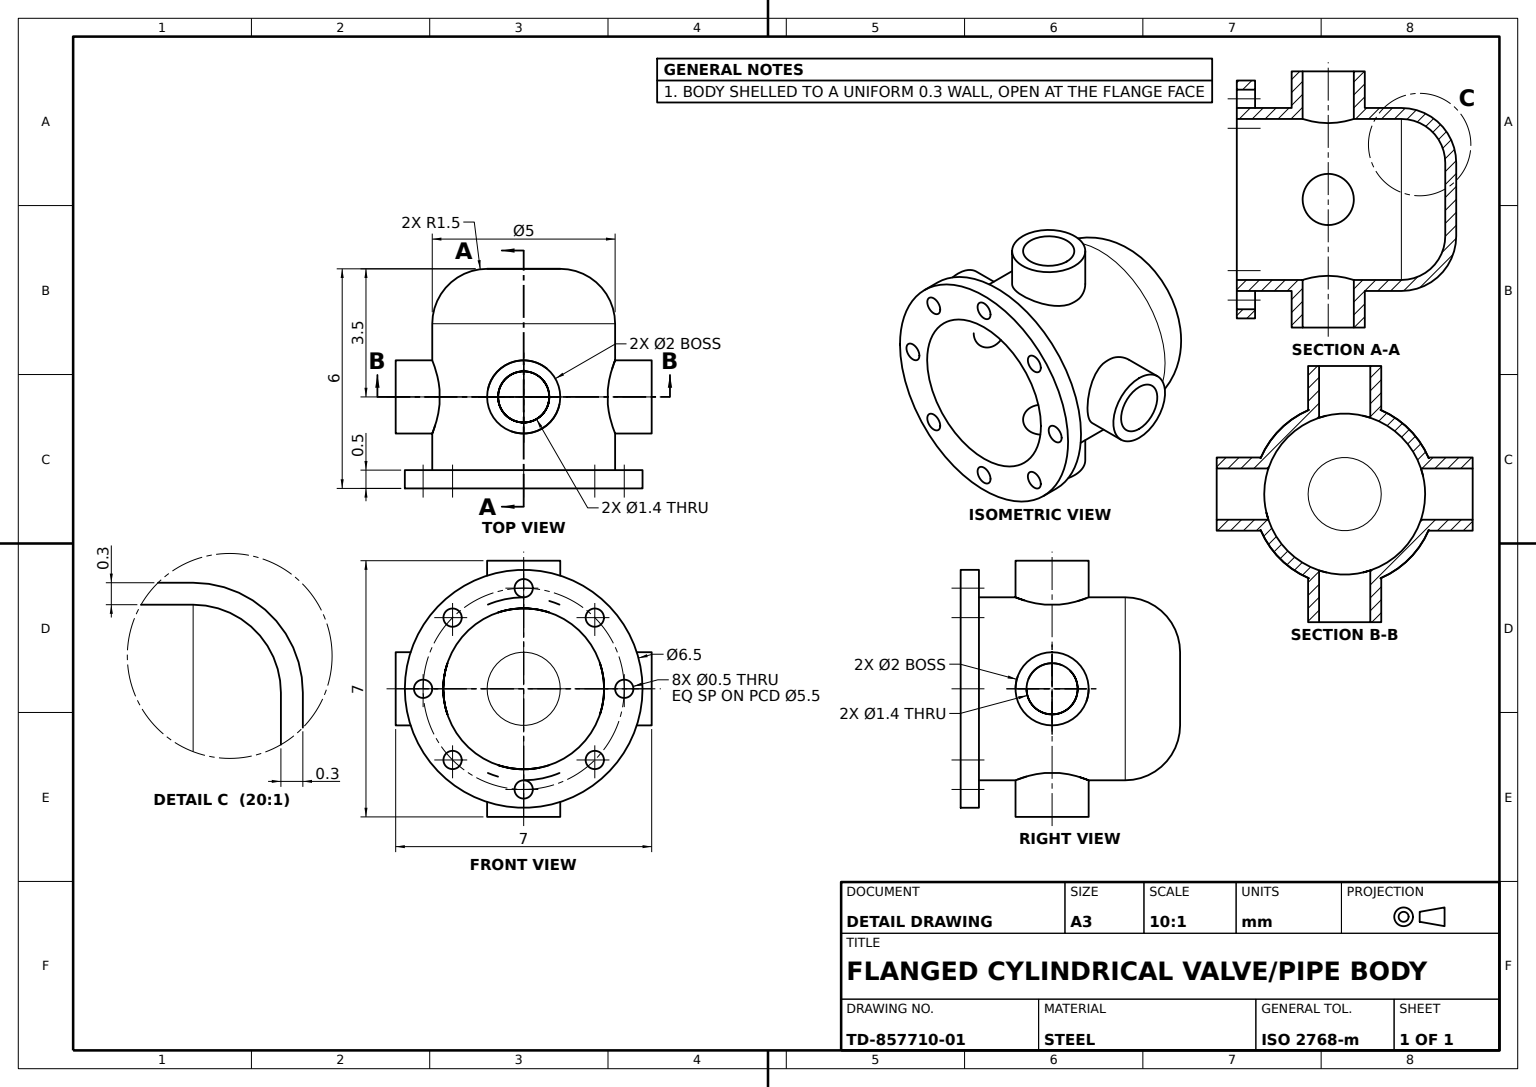
from build123d import *

# Parameters (mm, degrees)
BODY_SHELL_0_3_T            = -0.3
FLANGE_SKETCH_6_5_R         = 3.25
FLANGE_DEPTH                = 0.5
FLANGE_START                = -0.5
FLANGE_BORE_SKETCH_R        = 2.2
FLANGE_BORE_DEPTH           = 0.5
FLANGE_BOLT_HOLES_SKETCH_R  = 0.25
FLANGE_BOLT_HOLES_8X_DEPTH  = 0.5
SIDE_PORT_BOSS_SKETCH_2_R   = 1
SIDE_PORT_BOSS_DEPTH        = 1.2
SIDE_PORT_BORE_SKETCH_1_4_R = 0.7
SIDE_PORT_BORE_1_4_DEPTH    = 1.5
SIDE_PORT_PATTERN_4X_COUNT  = 4


with BuildPart() as part:
    # Body Profile Sketch → Body Revolve (revolve)
    with BuildSketch(Plane.XY, mode=Mode.PRIVATE) as body_revolve_sk:
        with BuildLine():
            Line((0, 0), (0, 5.5))
            Line((0, 5.5), (-2.5, 5.5))
            Line((-2.5, 5.5), (-2.5, 1.5))
            ThreePointArc((-2.5, 1.5), (-2.060660172, 0.439339828), (-1, 0))
            Line((-1, 0), (0, 0))
        make_face()
    revolve(body_revolve_sk.sketch.rotate(Axis((0, 0, 0), (0, 1, 0)), 270), axis=Axis((0, 0, 0), (0, 1, 0)))

    # Body Shell 0.3
    body_shell_0_3_openings = [part.faces().sort_by_distance(p)[0] for p in [
        (0, 5.5, 0),
    ]]
    offset(amount=BODY_SHELL_0_3_T, openings=body_shell_0_3_openings, kind=Kind.INTERSECTION)

    # Flange Sketch Ø6.5 → Flange (add)
    with BuildSketch(Plane(origin=(0, 5.5, 0), x_dir=(1, 0, 0), z_dir=(0, 1, 0))):
        with Locations(Location((0, 0, 0), (0, 0, 270))):
            Circle(FLANGE_SKETCH_6_5_R)
    extrude(amount=FLANGE_DEPTH)

    # Flange Bore Sketch → Flange Bore (cut)
    with BuildSketch(Plane(origin=(0, 6, 0), x_dir=(1, 0, 0), z_dir=(0, 1, 0)).offset(FLANGE_START)):
        with Locations(Location((0, 0, 0), (0, 0, 90))):
            Circle(FLANGE_BORE_SKETCH_R)
    extrude(amount=FLANGE_BORE_DEPTH, mode=Mode.SUBTRACT)

    # Flange Bolt Holes Sketch → Flange Bolt Holes 8x (cut)
    with BuildSketch(Plane(origin=(0, 6, 0), x_dir=(1, 0, 0), z_dir=(0, 1, 0))):
        with Locations(Location((0, 2.75, 0), (0, 0, 270))):
            Circle(FLANGE_BOLT_HOLES_SKETCH_R)
        with Locations(Location((1.944543648, 1.944543648, 0), (0, 0, 270))):
            Circle(FLANGE_BOLT_HOLES_SKETCH_R)
        with Locations(Location((2.75, 0, 0), (0, 0, 270))):
            Circle(FLANGE_BOLT_HOLES_SKETCH_R)
        with Locations(Location((1.944543648, -1.944543648, 0), (0, 0, 270))):
            Circle(FLANGE_BOLT_HOLES_SKETCH_R)
        with Locations(Location((0, -2.75, 0), (0, 0, 270))):
            Circle(FLANGE_BOLT_HOLES_SKETCH_R)
        with Locations(Location((-1.944543648, -1.944543648, 0), (0, 0, 270))):
            Circle(FLANGE_BOLT_HOLES_SKETCH_R)
        with Locations(Location((-2.75, 0, 0), (0, 0, 270))):
            Circle(FLANGE_BOLT_HOLES_SKETCH_R)
        with Locations(Location((-1.944543648, 1.944543648, 0), (0, 0, 270))):
            Circle(FLANGE_BOLT_HOLES_SKETCH_R)
    extrude(amount=-FLANGE_BOLT_HOLES_8X_DEPTH, mode=Mode.SUBTRACT)

    # Side Port Boss Sketch Ø2 → Side Port Boss (add)
    with BuildSketch(Plane.XY.offset(3.5)):
        with Locations((0, 3.5)):
            Circle(SIDE_PORT_BOSS_SKETCH_2_R)
    side_port_boss = extrude(amount=-SIDE_PORT_BOSS_DEPTH)

    # Side Port Bore Sketch Ø1.4 → Side Port Bore Ø1.4 (cut)
    with BuildSketch(Plane.XY.offset(3.5)):
        with Locations((0, 3.5)):
            Circle(SIDE_PORT_BORE_SKETCH_1_4_R)
    side_port_bore_1_4 = extrude(amount=-SIDE_PORT_BORE_1_4_DEPTH, mode=Mode.SUBTRACT)

    # Side Port Pattern 4x: Side Port Boss, Side Port Bore Ø1.4 ×4 about axis
    side_port_pattern_4x_axis = Axis((0, 0, 0), (0, 1, 0))
    add([side_port_boss.rotate(side_port_pattern_4x_axis, i * 360 / SIDE_PORT_PATTERN_4X_COUNT) for i in range(1, SIDE_PORT_PATTERN_4X_COUNT)])
    add([side_port_bore_1_4.rotate(side_port_pattern_4x_axis, i * 360 / SIDE_PORT_PATTERN_4X_COUNT) for i in range(1, SIDE_PORT_PATTERN_4X_COUNT)], mode=Mode.SUBTRACT)


solid = part.part
